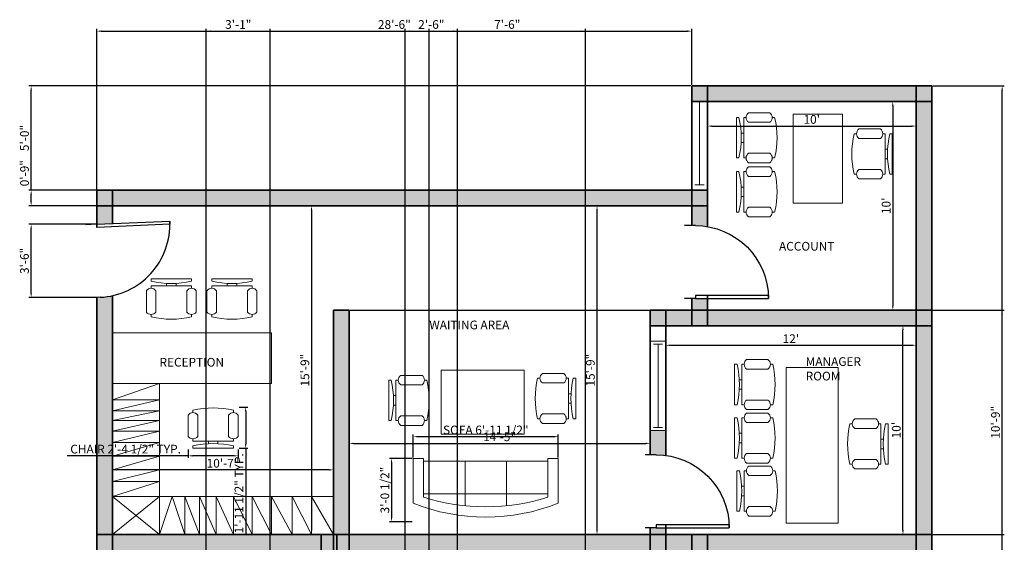
# Model space of a CAD drawing. Units: millimetres. Extents: x 2436 to 3005, y 774 to 1472.
# Tile 3 of 3: x 2436 to 3002, y 1172 to 1472. Entities that reach past the tile are written whole.
import ezdxf

# ---------------------------------------------------------------- set-up
doc = ezdxf.new("R2010")
doc.units = ezdxf.units.MM
for name, color, linetype, lineweight in [('A-ANNO-DIMS', 2, 'Continuous', 18), ('A-AREA-IDEN', 10, 'Continuous', 25), ('A-FLOR-CASE', 140, 'Continuous', 18), ('A-WALL-PATT', 3, 'Continuous', 13), ('doors', 30, 'Continuous', 25), ('furniture', 140, 'Continuous', 18), ('walls', 80, 'Continuous', 35), ('window', 190, 'Continuous', 20)]:
    doc.layers.add(name, color=color, linetype=linetype, lineweight=lineweight)
doc.styles.get("Standard").update_dxf_attribs({"font": 'arial.ttf'})
doc.dimstyles.new('ISO-25', dxfattribs={"dimtxt": 5, "dimasz": 2.5, "dimexe": 1.25, "dimexo": 0.625, "dimtad": 1, "dimdec": 0, "dimlunit": 3, "dimtxsty": 'Standard', "dimcen": 2.5, "dimadec": 0, "dimazin": 0, "dimtfac": 1, "dimtdec": 0, "dimtmove": 0, "dimatfit": 3, "dimfxl": 1, "dimarcsym": 0})

# ---------------------------------------------------------------- blocks, each defined once
blk = doc.blocks.new('*U2')
for p, q in [((0, 0), (0, -6)), ((40, 0), (40, -6))]:
    blk.add_line(p, q)
blk.add_lwpolyline([(0, 0), (0, 40), (1.75, 40), (1.75, 0)], close=True)
blk.add_arc((0, 0), 40, 0, 90)
blk = doc.blocks.new('*U4')
for p, q in [((0, 4), (0, 0)), ((0, 2), (36, 2)), ((36, 4), (36, 0))]:
    blk.add_line(p, q)
blk = doc.blocks.new('Sofa - Roundback 7 ft.')
for p, q in [((-12.00002, -32.4421), (-12.00003, -6.5971)), ((11.99997, -32.4421), (11.99998, -6.5971)), ((-36.000027, -34), (-36.000027, -11.4696)), ((-35.999844, -13.3819), (35.9998, -13.3819)), ((35.99998, -34), (35.99998, -11.4696)), ((-36.000027, -32.4421), (35.99998, -32.4421))]:
    blk.add_line(p, q)
for points in [[(-36.000027, -34), (-42.000027, -34), (-42.000027, -8)], [(41.99998, -8), (41.99998, -34), (35.99998, -34)]]:
    blk.add_lwpolyline(points)
for centre, radius, start, end in [((0, -114.25), 114.25, 68.43141, 111.5686), ((-0.00001, -127.1968), 121.1968, 72.72033, 107.2797)]:
    blk.add_arc(centre, radius, start, end)
blk = doc.blocks.new('Chair - Desk')
for p, q in [((-8.5, 0), (-8.5, -1)), ((-8.5, 0), (8.5, 0)), ((8.5, 0), (8.5, -1)), ((-8.5, -3), (-8.5, -4)), ((-8.5, -3), (8.5, -3)), ((-2, -3), (-2, -1.9355)), ((2, -1.9576), (2, -3)), ((8.5, -3), (8.5, -4)), ((-10.5, -5), (-10.5, -14)), ((-6.5, -14), (-6.5, -5)), ((6.5, -5), (6.5, -14)), ((10.5, -14), (10.5, -5)), ((-8.5, -15), (-8.5, -16)), ((8.5, -15), (8.5, -16))]:
    blk.add_line(p, q)
for centre, radius, start, end in [((-8.5, -6.5), 2.5, 36.8699, 143.1301), ((0, 34.625), 36.625, 256.5803, 283.4197), ((8.5, -6.5), 2.5, 36.8699, 143.1301), ((-8.5, -12.5), 2.5, 216.8699, 323.1301), ((0, 19.625), 36.625, 256.5803, 283.4197), ((8.5, -12.5), 2.5, 216.8699, 323.1301)]:
    blk.add_arc(centre, radius, start, end)
blk = doc.blocks.new('*D9')
at = {"layer": 'A-ANNO-DIMS', "color": 0, "lineweight": -2, "transparency": 16777216}
for p, q in [((2601.07, 1365.12), (2604.93, 1365.12)), ((2603.68, 1362.62), (2603.68, 1178.62)), ((2604.3, 1176.12), (2604.93, 1176.12))]:
    blk.add_line(p, q, dxfattribs=at)
at = {"layer": 'A-ANNO-DIMS', "color": 0, "transparency": 16777216}
for points in [[(2603.26, 1362.62), (2604.09, 1362.62), (2603.68, 1365.12)], [(2603.26, 1178.62), (2604.09, 1178.62), (2603.68, 1176.12)]]:
    blk.add_solid(points, dxfattribs=at)
at = {"layer": 'Defpoints', "color": 0, "transparency": 16777216}
for p in [(2600.44, 1365.12), (2603.68, 1176.12), (2603.68, 1176.12)]:
    blk.add_point(p, dxfattribs=at)
at = {"layer": 'A-ANNO-DIMS', "color": 0, "transparency": 16777216, "insert": (2600.5, 1270.62), "char_height": 5, "attachment_point": 5, "rotation": 90}
blk.add_mtext('15\'-9"', dxfattribs=at)
blk = doc.blocks.new('*D10')
at = {"layer": 'A-ANNO-DIMS', "color": 0, "lineweight": -2, "transparency": 16777216}
for p, q in [((2489.3, 1218.94), (2489.3, 1212.03)), ((2613.8, 1213.28), (2491.8, 1213.28)), ((2616.3, 1215.03), (2616.3, 1212.03))]:
    blk.add_line(p, q, dxfattribs=at)
at = {"layer": 'A-ANNO-DIMS', "color": 0, "transparency": 16777216}
for points in [[(2491.8, 1213.7), (2491.8, 1212.87), (2489.3, 1213.28)], [(2613.8, 1213.7), (2613.8, 1212.87), (2616.3, 1213.28)]]:
    blk.add_solid(points, dxfattribs=at)
at = {"layer": 'Defpoints', "color": 0, "transparency": 16777216}
for p in [(2489.3, 1219.57), (2489.3, 1213.28), (2616.3, 1215.66)]:
    blk.add_point(p, dxfattribs=at)
at = {"layer": 'A-ANNO-DIMS', "color": 0, "transparency": 16777216, "insert": (2552.8, 1216.46), "char_height": 5, "attachment_point": 5}
blk.add_mtext('10\'-7"', dxfattribs=at)
blk = doc.blocks.new('*D11')
at = {"layer": 'A-ANNO-DIMS', "color": 0, "lineweight": -2, "transparency": 16777216}
for p, q in [((2625.3, 1229.12), (2625.3, 1229.75)), ((2627.8, 1228.5), (2795.8, 1228.5)), ((2798.3, 1229.12), (2798.3, 1229.75))]:
    blk.add_line(p, q, dxfattribs=at)
at = {"layer": 'A-ANNO-DIMS', "color": 0, "transparency": 16777216}
for points in [[(2627.8, 1228.91), (2627.8, 1228.08), (2625.3, 1228.5)], [(2795.8, 1228.91), (2795.8, 1228.08), (2798.3, 1228.5)]]:
    blk.add_solid(points, dxfattribs=at)
at = {"layer": 'Defpoints', "color": 0, "transparency": 16777216}
for p in [(2625.3, 1228.5), (2798.3, 1228.5), (2798.3, 1228.5)]:
    blk.add_point(p, dxfattribs=at)
at = {"layer": 'A-ANNO-DIMS', "color": 0, "transparency": 16777216, "insert": (2711.8, 1231.67), "char_height": 5, "attachment_point": 5}
blk.add_mtext('14\'-5"', dxfattribs=at)
blk = doc.blocks.new('*D12')
at = {"layer": 'A-ANNO-DIMS', "color": 0, "lineweight": -2, "transparency": 16777216}
for p, q in [((2773.45, 1365.12), (2766.59, 1365.12)), ((2767.84, 1178.62), (2767.84, 1362.62)), ((2773.45, 1176.12), (2766.59, 1176.12))]:
    blk.add_line(p, q, dxfattribs=at)
at = {"layer": 'A-ANNO-DIMS', "color": 0, "transparency": 16777216}
for points in [[(2767.42, 1362.62), (2768.25, 1362.62), (2767.84, 1365.12)], [(2767.42, 1178.62), (2768.25, 1178.62), (2767.84, 1176.12)]]:
    blk.add_solid(points, dxfattribs=at)
at = {"layer": 'Defpoints', "color": 0, "transparency": 16777216}
for p in [(2767.84, 1365.12), (2774.07, 1365.12), (2774.07, 1176.12)]:
    blk.add_point(p, dxfattribs=at)
at = {"layer": 'A-ANNO-DIMS', "color": 0, "transparency": 16777216, "insert": (2764.66, 1270.62), "char_height": 5, "attachment_point": 5, "rotation": 90}
blk.add_mtext('15\'-9"', dxfattribs=at)
blk = doc.blocks.new('*D13')
at = {"layer": 'A-ANNO-DIMS', "color": 0, "lineweight": -2, "transparency": 16777216}
for p, q in [((2807.3, 1286.74), (2807.3, 1283.69)), ((2951.3, 1286.74), (2951.3, 1283.69)), ((2809.8, 1284.94), (2948.8, 1284.94))]:
    blk.add_line(p, q, dxfattribs=at)
at = {"layer": 'A-ANNO-DIMS', "color": 0, "transparency": 16777216}
for points in [[(2809.8, 1285.36), (2809.8, 1284.53), (2807.3, 1284.94)], [(2948.8, 1285.36), (2948.8, 1284.53), (2951.3, 1284.94)]]:
    blk.add_solid(points, dxfattribs=at)
at = {"layer": 'Defpoints', "color": 0, "transparency": 16777216}
for p in [(2807.3, 1287.36), (2951.3, 1287.36), (2951.3, 1284.94)]:
    blk.add_point(p, dxfattribs=at)
at = {"layer": 'A-ANNO-DIMS', "color": 0, "transparency": 16777216, "insert": (2879.3, 1288.08), "char_height": 5, "attachment_point": 5}
blk.add_mtext("12'", dxfattribs=at)
blk = doc.blocks.new('*D14')
at = {"layer": 'A-ANNO-DIMS', "color": 0, "lineweight": -2, "transparency": 16777216}
for p, q in [((2943.72, 1178.62), (2943.72, 1293.62)), ((2944.34, 1296.12), (2944.97, 1296.12)), ((2944.34, 1176.12), (2944.97, 1176.12))]:
    blk.add_line(p, q, dxfattribs=at)
at = {"layer": 'A-ANNO-DIMS', "color": 0, "transparency": 16777216}
for points in [[(2943.3, 1293.62), (2944.14, 1293.62), (2943.72, 1296.12)], [(2943.3, 1178.62), (2944.14, 1178.62), (2943.72, 1176.12)]]:
    blk.add_solid(points, dxfattribs=at)
at = {"layer": 'Defpoints', "color": 0, "transparency": 16777216}
for p in [(2943.72, 1296.12), (2943.72, 1296.12), (2943.72, 1176.12)]:
    blk.add_point(p, dxfattribs=at)
at = {"layer": 'A-ANNO-DIMS', "color": 0, "transparency": 16777216, "insert": (2940.54, 1236.12), "char_height": 5, "attachment_point": 5, "rotation": 90}
blk.add_mtext("10'", dxfattribs=at)
blk = doc.blocks.new('*D15')
at = {"layer": 'A-ANNO-DIMS', "color": 0, "lineweight": -2, "transparency": 16777216}
for p, q in [((2937.9, 1422.62), (2937.9, 1307.62)), ((2938.53, 1425.12), (2939.15, 1425.12)), ((2938.53, 1305.12), (2939.15, 1305.12))]:
    blk.add_line(p, q, dxfattribs=at)
at = {"layer": 'A-ANNO-DIMS', "color": 0, "transparency": 16777216}
for points in [[(2937.48, 1422.62), (2938.32, 1422.62), (2937.9, 1425.12)], [(2937.48, 1307.62), (2938.32, 1307.62), (2937.9, 1305.12)]]:
    blk.add_solid(points, dxfattribs=at)
at = {"layer": 'Defpoints', "color": 0, "transparency": 16777216}
for p in [(2937.9, 1425.12), (2937.9, 1305.12), (2937.9, 1305.12)]:
    blk.add_point(p, dxfattribs=at)
at = {"layer": 'A-ANNO-DIMS', "color": 0, "transparency": 16777216, "insert": (2934.72, 1365.12), "char_height": 5, "attachment_point": 5, "rotation": 90}
blk.add_mtext("10'", dxfattribs=at)
blk = doc.blocks.new('*D16')
at = {"layer": 'A-ANNO-DIMS', "color": 0, "lineweight": -2, "transparency": 16777216}
for p, q in [((2831.3, 1411.6), (2831.3, 1412.23)), ((2833.8, 1410.98), (2948.8, 1410.98)), ((2951.3, 1411.6), (2951.3, 1412.23))]:
    blk.add_line(p, q, dxfattribs=at)
at = {"layer": 'A-ANNO-DIMS', "color": 0, "transparency": 16777216}
for points in [[(2833.8, 1411.39), (2833.8, 1410.56), (2831.3, 1410.98)], [(2948.8, 1411.39), (2948.8, 1410.56), (2951.3, 1410.98)]]:
    blk.add_solid(points, dxfattribs=at)
at = {"layer": 'Defpoints', "color": 0, "transparency": 16777216}
for p in [(2831.3, 1410.98), (2951.3, 1410.98), (2951.3, 1410.98)]:
    blk.add_point(p, dxfattribs=at)
at = {"layer": 'A-ANNO-DIMS', "color": 0, "transparency": 16777216, "insert": (2891.3, 1414.15), "char_height": 5, "attachment_point": 5}
blk.add_mtext("10'", dxfattribs=at)
blk = doc.blocks.new('*D34')
at = {"layer": 'A-ANNO-DIMS', "color": 0, "lineweight": -2, "transparency": 16777216}
for p, q in [((2532.76, 1225.04), (2532.76, 1220.11)), ((2561.51, 1225.04), (2561.51, 1220.11)), ((2532.76, 1221.36), (2463.27, 1221.36)), ((2559.01, 1221.36), (2535.26, 1221.36))]:
    blk.add_line(p, q, dxfattribs=at)
at = {"layer": 'A-ANNO-DIMS', "color": 0, "transparency": 16777216}
for points in [[(2535.26, 1221.77), (2535.26, 1220.94), (2532.76, 1221.36)], [(2559.01, 1221.77), (2559.01, 1220.94), (2561.51, 1221.36)]]:
    blk.add_solid(points, dxfattribs=at)
at = {"layer": 'Defpoints', "color": 0, "transparency": 16777216}
for p in [(2532.76, 1225.67), (2561.51, 1225.67), (2532.76, 1221.36)]:
    blk.add_point(p, dxfattribs=at)
at = {"layer": 'A-ANNO-DIMS', "color": 0, "transparency": 16777216, "insert": (2496.77, 1224.57), "char_height": 5, "attachment_point": 5}
blk.add_mtext('CHAIR 2\'-4 1/2" TYP.', dxfattribs=at)
blk = doc.blocks.new('*D35')
at = {"layer": 'A-ANNO-DIMS', "color": 0, "lineweight": -2, "transparency": 16777216}
for p, q in [((2562.13, 1249.39), (2567.07, 1249.39)), ((2565.82, 1246.89), (2565.82, 1228.17)), ((2562.13, 1225.67), (2567.07, 1225.67)), ((2565.82, 1225.67), (2565.82, 1176.38))]:
    blk.add_line(p, q, dxfattribs=at)
at = {"layer": 'A-ANNO-DIMS', "color": 0, "transparency": 16777216}
for points in [[(2565.4, 1246.89), (2566.23, 1246.89), (2565.82, 1249.39)], [(2565.4, 1228.17), (2566.23, 1228.17), (2565.82, 1225.67)]]:
    blk.add_solid(points, dxfattribs=at)
at = {"layer": 'Defpoints', "color": 0, "transparency": 16777216}
for p in [(2561.51, 1249.39), (2561.51, 1225.67), (2565.82, 1225.67)]:
    blk.add_point(p, dxfattribs=at)
at = {"layer": 'A-ANNO-DIMS', "color": 0, "transparency": 16777216, "insert": (2562.61, 1199.77), "char_height": 5, "attachment_point": 5, "rotation": 90}
blk.add_mtext('1\'-11 1/2" TYP.', dxfattribs=at)
blk = doc.blocks.new('*D38')
at = {"layer": 'A-ANNO-DIMS', "color": 0, "lineweight": -2, "transparency": 16777216}
for p, q in [((2662.2, 1220.49), (2662.2, 1233.62)), ((2743.04, 1232.37), (2664.7, 1232.37)), ((2745.54, 1220.49), (2745.54, 1233.62))]:
    blk.add_line(p, q, dxfattribs=at)
at = {"layer": 'A-ANNO-DIMS', "color": 0, "transparency": 16777216}
for points in [[(2664.7, 1232.79), (2664.7, 1231.95), (2662.2, 1232.37)], [(2743.04, 1232.79), (2743.04, 1231.95), (2745.54, 1232.37)]]:
    blk.add_solid(points, dxfattribs=at)
at = {"layer": 'Defpoints', "color": 0, "transparency": 16777216}
for p in [(2662.2, 1232.37), (2662.2, 1219.87), (2745.54, 1219.87)]:
    blk.add_point(p, dxfattribs=at)
at = {"layer": 'A-ANNO-DIMS', "color": 0, "transparency": 16777216, "insert": (2703.87, 1235.58), "char_height": 5, "attachment_point": 5}
blk.add_mtext('SOFA 6\'-11 1/2"', dxfattribs=at)
blk = doc.blocks.new('*D39')
at = {"layer": 'A-ANNO-DIMS', "color": 0, "lineweight": -2, "transparency": 16777216}
for p, q in [((2661.57, 1219.87), (2648.45, 1219.87)), ((2649.7, 1217.37), (2649.7, 1185.99)), ((2661.57, 1183.49), (2648.45, 1183.49))]:
    blk.add_line(p, q, dxfattribs=at)
at = {"layer": 'A-ANNO-DIMS', "color": 0, "transparency": 16777216}
for points in [[(2649.28, 1217.37), (2650.11, 1217.37), (2649.7, 1219.87)], [(2649.28, 1185.99), (2650.11, 1185.99), (2649.7, 1183.49)]]:
    blk.add_solid(points, dxfattribs=at)
at = {"layer": 'Defpoints', "color": 0, "transparency": 16777216}
for p in [(2662.2, 1219.87), (2649.7, 1183.49), (2662.2, 1183.49)]:
    blk.add_point(p, dxfattribs=at)
at = {"layer": 'A-ANNO-DIMS', "color": 0, "transparency": 16777216, "insert": (2646.48, 1201.68), "char_height": 5, "attachment_point": 5, "rotation": 90}
blk.add_mtext('3\'-0 1/2"', dxfattribs=at)
blk = doc.blocks.new('*D41')
at = {"layer": 'A-ANNO-DIMS', "color": 0, "lineweight": -2, "transparency": 16777216}
for p, q in [((2960.92, 1434.12), (3002, 1434.12)), ((3000.75, 809.62), (3000.75, 1431.62)), ((2969.92, 807.12), (3002, 807.12))]:
    blk.add_line(p, q, dxfattribs=at)
at = {"layer": 'A-ANNO-DIMS', "color": 0, "transparency": 16777216}
for points in [[(3000.33, 1431.62), (3001.17, 1431.62), (3000.75, 1434.12)], [(3000.33, 809.62), (3001.17, 809.62), (3000.75, 807.12)]]:
    blk.add_solid(points, dxfattribs=at)
at = {"layer": 'Defpoints', "color": 0, "transparency": 16777216}
for p in [(2960.3, 1434.12), (3000.75, 1434.12), (2969.3, 807.12)]:
    blk.add_point(p, dxfattribs=at)
at = {"layer": 'A-ANNO-DIMS', "color": 0, "transparency": 16777216, "insert": (2997.57, 1120.62), "char_height": 5, "attachment_point": 5, "rotation": 90}
blk.add_mtext('52\'-3"', dxfattribs=at)
blk = doc.blocks.new('*D43')
at = {"layer": 'A-ANNO-DIMS', "color": 0, "lineweight": -2, "transparency": 16777216}
for p, q in [((2822.3, 1175.5), (2822.3, 774.42)), ((2618.3, 1160.31), (2618.3, 774.42)), ((2620.8, 775.67), (2819.8, 775.67))]:
    blk.add_line(p, q, dxfattribs=at)
at = {"layer": 'A-ANNO-DIMS', "color": 0, "transparency": 16777216}
for points in [[(2620.8, 776.09), (2620.8, 775.26), (2618.3, 775.67)], [(2819.8, 776.09), (2819.8, 775.26), (2822.3, 775.67)]]:
    blk.add_solid(points, dxfattribs=at)
at = {"layer": 'Defpoints', "color": 0, "transparency": 16777216}
for p in [(2822.3, 1176.12), (2618.3, 1160.93), (2822.3, 775.67)]:
    blk.add_point(p, dxfattribs=at)
at = {"layer": 'A-ANNO-DIMS', "color": 0, "transparency": 16777216, "insert": (2720.3, 778.85), "char_height": 5, "attachment_point": 5}
blk.add_mtext('17\'-0"', dxfattribs=at)
blk = doc.blocks.new('*D45')
at = {"layer": 'A-ANNO-DIMS', "color": 0, "lineweight": -2, "transparency": 16777216}
for p, q in [((2480.3, 1374.75), (2480.3, 1466.82)), ((2822.3, 1434.75), (2822.3, 1466.82)), ((2482.8, 1465.57), (2819.8, 1465.57))]:
    blk.add_line(p, q, dxfattribs=at)
at = {"layer": 'A-ANNO-DIMS', "color": 0, "transparency": 16777216}
for points in [[(2482.8, 1465.99), (2482.8, 1465.16), (2480.3, 1465.57)], [(2819.8, 1465.99), (2819.8, 1465.16), (2822.3, 1465.57)]]:
    blk.add_solid(points, dxfattribs=at)
at = {"layer": 'Defpoints', "color": 0, "transparency": 16777216}
for p in [(2822.3, 1465.57), (2822.3, 1434.12), (2480.3, 1374.12)]:
    blk.add_point(p, dxfattribs=at)
at = {"layer": 'A-ANNO-DIMS', "color": 0, "transparency": 16777216, "insert": (2651.3, 1468.75), "char_height": 5, "attachment_point": 5}
blk.add_mtext('28\'-6"', dxfattribs=at)
blk = doc.blocks.new('*D46')
at = {"layer": 'A-ANNO-DIMS', "color": 0, "lineweight": -2, "transparency": 16777216}
for p, q in [((2821.67, 1434.12), (2441.22, 1434.12)), ((2442.47, 1376.62), (2442.47, 1431.62)), ((2830.67, 1374.12), (2441.22, 1374.12))]:
    blk.add_line(p, q, dxfattribs=at)
at = {"layer": 'A-ANNO-DIMS', "color": 0, "transparency": 16777216}
for points in [[(2442.06, 1431.62), (2442.89, 1431.62), (2442.47, 1434.12)], [(2442.06, 1376.62), (2442.89, 1376.62), (2442.47, 1374.12)]]:
    blk.add_solid(points, dxfattribs=at)
at = {"layer": 'Defpoints', "color": 0, "transparency": 16777216}
for p in [(2442.47, 1434.12), (2822.3, 1434.12), (2831.3, 1374.12)]:
    blk.add_point(p, dxfattribs=at)
at = {"layer": 'A-ANNO-DIMS', "color": 0, "transparency": 16777216, "insert": (2439.29, 1404.12), "char_height": 5, "attachment_point": 5, "rotation": 90}
blk.add_mtext('5\'-0"', dxfattribs=at)
blk = doc.blocks.new('*D47')
at = {"layer": 'A-ANNO-DIMS', "color": 0, "lineweight": -2, "transparency": 16777216}
for p, q in [((2479.59, 1354.48), (2441.22, 1354.48)), ((2442.47, 1314.94), (2442.47, 1351.98)), ((2479.67, 1312.44), (2441.22, 1312.44))]:
    blk.add_line(p, q, dxfattribs=at)
at = {"layer": 'A-ANNO-DIMS', "color": 0, "transparency": 16777216}
for points in [[(2442.06, 1351.98), (2442.89, 1351.98), (2442.47, 1354.48)], [(2442.06, 1314.94), (2442.89, 1314.94), (2442.47, 1312.44)]]:
    blk.add_solid(points, dxfattribs=at)
at = {"layer": 'Defpoints', "color": 0, "transparency": 16777216}
for p in [(2442.47, 1354.48), (2480.22, 1354.48), (2480.3, 1312.44)]:
    blk.add_point(p, dxfattribs=at)
at = {"layer": 'A-ANNO-DIMS', "color": 0, "transparency": 16777216, "insert": (2439.29, 1333.46), "char_height": 5, "attachment_point": 5, "rotation": 90}
blk.add_mtext('3\'-6"', dxfattribs=at)
blk = doc.blocks.new('*D48')
at = {"layer": 'A-ANNO-DIMS', "color": 0, "lineweight": -2, "transparency": 16777216}
for p, q in [((2442.47, 1374.12), (2442.47, 1391.16)), ((2479.67, 1374.12), (2441.22, 1374.12)), ((2442.47, 1367.62), (2442.47, 1371.62)), ((2479.67, 1365.12), (2441.22, 1365.12))]:
    blk.add_line(p, q, dxfattribs=at)
at = {"layer": 'A-ANNO-DIMS', "color": 0, "transparency": 16777216}
for points in [[(2442.06, 1371.62), (2442.89, 1371.62), (2442.47, 1374.12)], [(2442.06, 1367.62), (2442.89, 1367.62), (2442.47, 1365.12)]]:
    blk.add_solid(points, dxfattribs=at)
at = {"layer": 'Defpoints', "color": 0, "transparency": 16777216}
for p in [(2442.47, 1374.12), (2480.3, 1374.12), (2480.3, 1365.12)]:
    blk.add_point(p, dxfattribs=at)
at = {"layer": 'A-ANNO-DIMS', "color": 0, "transparency": 16777216, "insert": (2439.29, 1383.89), "char_height": 5, "attachment_point": 5, "rotation": 90}
blk.add_mtext('0\'-9"', dxfattribs=at)
blk = doc.blocks.new('*D49')
at = {"layer": 'A-ANNO-DIMS', "color": 0, "lineweight": -2, "transparency": 16777216}
for p, q in [((2671.31, 1103.79), (2671.31, 1466.82)), ((2761.12, 1103.79), (2761.12, 1466.82)), ((2673.81, 1465.57), (2758.62, 1465.57))]:
    blk.add_line(p, q, dxfattribs=at)
at = {"layer": 'A-ANNO-DIMS', "color": 0, "transparency": 16777216}
for points in [[(2673.81, 1465.99), (2673.81, 1465.16), (2671.31, 1465.57)], [(2758.62, 1465.99), (2758.62, 1465.16), (2761.12, 1465.57)]]:
    blk.add_solid(points, dxfattribs=at)
at = {"layer": 'Defpoints', "color": 0, "transparency": 16777216}
for p in [(2761.12, 1465.57), (2671.31, 1103.17), (2761.12, 1103.17)]:
    blk.add_point(p, dxfattribs=at)
at = {"layer": 'A-ANNO-DIMS', "color": 0, "transparency": 16777216, "insert": (2716.21, 1468.75), "char_height": 5, "attachment_point": 5}
blk.add_mtext('7\'-6"', dxfattribs=at)
blk = doc.blocks.new('*D51')
at = {"layer": 'A-ANNO-DIMS', "color": 0, "lineweight": -2, "transparency": 16777216}
for p, q in [((2625.92, 1305.12), (3002, 1305.12)), ((3000.75, 1178.62), (3000.75, 1302.62)), ((2618.92, 1176.12), (3002, 1176.12))]:
    blk.add_line(p, q, dxfattribs=at)
at = {"layer": 'A-ANNO-DIMS', "color": 0, "transparency": 16777216}
for points in [[(3000.33, 1302.62), (3001.17, 1302.62), (3000.75, 1305.12)], [(3000.33, 1178.62), (3001.17, 1178.62), (3000.75, 1176.12)]]:
    blk.add_solid(points, dxfattribs=at)
at = {"layer": 'Defpoints', "color": 0, "transparency": 16777216}
for p in [(2625.3, 1305.12), (3000.75, 1305.12), (2618.3, 1176.12)]:
    blk.add_point(p, dxfattribs=at)
at = {"layer": 'A-ANNO-DIMS', "color": 0, "transparency": 16777216, "insert": (2997.57, 1240.62), "char_height": 5, "attachment_point": 5, "rotation": 90}
blk.add_mtext('10\'-9"', dxfattribs=at)
blk = doc.blocks.new('*D52')
at = {"layer": 'A-ANNO-DIMS', "color": 0, "lineweight": -2, "transparency": 16777216}
for p, q in [((2657.55, 932.75), (2657.55, 1466.82)), ((2687.55, 932.75), (2687.55, 1466.82)), ((2660.05, 1465.57), (2685.05, 1465.57))]:
    blk.add_line(p, q, dxfattribs=at)
at = {"layer": 'A-ANNO-DIMS', "color": 0, "transparency": 16777216}
for points in [[(2660.05, 1465.99), (2660.05, 1465.16), (2657.55, 1465.57)], [(2685.05, 1465.99), (2685.05, 1465.16), (2687.55, 1465.57)]]:
    blk.add_solid(points, dxfattribs=at)
at = {"layer": 'Defpoints', "color": 0, "transparency": 16777216}
for p in [(2687.55, 1465.57), (2657.55, 932.12), (2687.55, 932.12)]:
    blk.add_point(p, dxfattribs=at)
at = {"layer": 'A-ANNO-DIMS', "color": 0, "transparency": 16777216, "insert": (2672.55, 1468.75), "char_height": 5, "attachment_point": 5}
blk.add_mtext('2\'-6"', dxfattribs=at)
blk = doc.blocks.new('*D53')
at = {"layer": 'A-ANNO-DIMS', "color": 0, "lineweight": -2, "transparency": 16777216}
for p, q in [((2543.16, 945.65), (2543.16, 1466.82)), ((2579.92, 945.65), (2579.92, 1466.82)), ((2545.66, 1465.57), (2577.42, 1465.57))]:
    blk.add_line(p, q, dxfattribs=at)
at = {"layer": 'A-ANNO-DIMS', "color": 0, "transparency": 16777216}
for points in [[(2545.66, 1465.99), (2545.66, 1465.16), (2543.16, 1465.57)], [(2577.42, 1465.99), (2577.42, 1465.16), (2579.92, 1465.57)]]:
    blk.add_solid(points, dxfattribs=at)
at = {"layer": 'Defpoints', "color": 0, "transparency": 16777216}
for p in [(2579.92, 1465.57), (2543.16, 945.02), (2579.92, 945.02)]:
    blk.add_point(p, dxfattribs=at)
at = {"layer": 'A-ANNO-DIMS', "color": 0, "transparency": 16777216, "insert": (2561.54, 1468.75), "char_height": 5, "attachment_point": 5}
blk.add_mtext('3\'-1"', dxfattribs=at)

msp = doc.modelspace()

# ---------------------------------------------------------------- hatches: boundary and pattern name
at = {"layer": 'A-WALL-PATT'}
h = msp.add_hatch(color=256, dxfattribs=at)
h.dxf.hatch_style = 1
h.paths.add_polyline_path([(2822.3, 1374.12), (2489.3, 1374.12), (2489.3, 1365.12), (2822.3, 1365.12)])
h.paths.add_polyline_path([(2831.3, 1374.12), (2822.3, 1374.12), (2822.3, 1365.12), (2831.3, 1365.12)])
h.paths.add_polyline_path([(2831.3, 1365.12), (2822.3, 1365.12), (2822.3, 1353.75), (2824.37, 1353.75, -0.041466), (2831.3, 1353.17)])
h.paths.add_polyline_path([(2960.3, 1425.12), (2951.3, 1425.12), (2951.3, 1305.12), (2960.3, 1305.12)])
h.paths.add_polyline_path([(2960.3, 1434.12), (2951.3, 1434.12), (2951.3, 1425.12), (2960.3, 1425.12)])
h.paths.add_polyline_path([(2951.3, 1434.12), (2831.3, 1434.12), (2831.3, 1425.12), (2951.3, 1425.12)])
h.paths.add_polyline_path([(2831.3, 1434.12), (2822.3, 1434.12), (2822.3, 1425.12), (2831.3, 1425.12)])
h.paths.add_polyline_path([(2489.3, 1374.12), (2480.3, 1374.12), (2480.3, 1365.12), (2489.3, 1365.12)])
h.paths.add_polyline_path([(2489.3, 1365.12), (2480.3, 1365.12), (2480.3, 1354.49), (2489.3, 1354.89)])
h.paths.add_polyline_path([(2489.3, 1313.48, -0.04329), (2482.1, 1312.53), (2480.3, 1312.44), (2480.3, 1176.12), (2489.3, 1176.12)])
h.paths.add_polyline_path([(2489.3, 1176.12), (2480.3, 1176.12), (2480.3, 1167.12), (2489.3, 1167.12)])
h.paths.add_polyline_path([(2609.3, 1176.12), (2489.3, 1176.12), (2489.3, 1167.12), (2609.3, 1167.12)])
h.paths.add_polyline_path([(2625.3, 1176.12), (2618.3, 1176.12), (2618.3, 1167.12), (2625.3, 1167.12)])
h.paths.add_polyline_path([(2618.3, 1176.12), (2616.3, 1176.12), (2616.3, 1167.12), (2618.3, 1167.12)])
h.paths.add_polyline_path([(2616.3, 1176.12), (2609.3, 1176.12), (2609.3, 1167.12), (2616.3, 1167.12)])
h.paths.add_polyline_path([(2618.3, 1167.12), (2609.3, 1167.12), (2609.3, 1160.63, -0.029892), (2614.31, 1160.93), (2618.3, 1160.93)])
h.paths.add_polyline_path([(2625.3, 1305.12), (2616.3, 1305.12), (2616.3, 1176.12), (2618.3, 1176.12), (2625.3, 1176.12)])
h.paths.add_polyline_path([(2798.3, 1176.12), (2625.3, 1176.12), (2625.3, 1167.12), (2798.3, 1167.12)])
h.paths.add_polyline_path([(2807.3, 1176.12), (2798.3, 1176.12), (2798.3, 1167.12), (2807.3, 1167.12)])
h.paths.add_polyline_path([(2831.3, 1176.12), (2822.3, 1176.12), (2822.3, 1167.12), (2831.3, 1167.12)])
h.paths.add_polyline_path([(2822.3, 1176.12), (2807.3, 1176.12), (2807.3, 1167.12), (2822.3, 1167.12)])
h.paths.add_polyline_path([(2951.3, 1176.12), (2831.3, 1176.12), (2831.3, 1167.12), (2951.3, 1167.12)])
h.paths.add_polyline_path([(2960.3, 1176.12), (2951.3, 1176.12), (2951.3, 1167.12), (2960.3, 1167.12)])
h.paths.add_polyline_path([(2960.3, 1296.12), (2951.3, 1296.12), (2951.3, 1176.12), (2960.3, 1176.12)])
h.paths.add_polyline_path([(2960.3, 1305.12), (2951.3, 1305.12), (2951.3, 1296.12), (2960.3, 1296.12)])
h.paths.add_polyline_path([(2951.3, 1305.12), (2831.3, 1305.12), (2831.3, 1296.12), (2951.3, 1296.12)])
h.paths.add_polyline_path([(2822.3, 1305.12), (2807.3, 1305.12), (2807.3, 1296.12), (2822.3, 1296.12)])
h.paths.add_polyline_path([(2831.3, 1305.12), (2822.3, 1305.12), (2822.3, 1296.12), (2831.3, 1296.12)])
h.paths.add_polyline_path([(2831.3, 1311.75), (2824.37, 1311.75), (2822.3, 1311.75), (2822.3, 1305.12), (2831.3, 1305.12)])
h.paths.add_polyline_path([(2807.3, 1305.12), (2798.3, 1305.12), (2798.3, 1296.12), (2807.3, 1296.12)])
h.paths.add_polyline_path([(2807.3, 1236.01), (2798.3, 1236.01), (2798.3, 1221.93), (2801.81, 1221.93, -0.032777), (2807.3, 1221.57)])
h.paths.add_polyline_path([(2831.3, 1167.12), (2822.3, 1167.12), (2822.3, 1139.2), (2826.09, 1139.2, -0.043681), (2831.3, 1138.75)])
h.paths.add_polyline_path([(2807.3, 1179.93), (2801.81, 1179.93), (2798.3, 1179.93), (2798.3, 1176.12), (2807.3, 1176.12)])
h.paths.add_polyline_path([(2927.3, 900.12), (2831.3, 900.12), (2831.3, 891.12), (2927.3, 891.12)])
h.paths.add_polyline_path([(2936.3, 900.12), (2927.3, 900.12), (2927.3, 891.12), (2936.3, 891.12)])
h.paths.add_polyline_path([(2936.3, 905.69), (2927.3, 905.69), (2927.3, 900.12), (2936.3, 900.12)])
h.paths.add_polyline_path([(2831.3, 900.12), (2822.3, 900.12), (2822.3, 891.12), (2831.3, 891.12)])
h.paths.add_polyline_path([(2831.3, 903.84), (2822.3, 903.84), (2822.3, 900.12), (2831.3, 900.12)])
h.paths.add_polyline_path([(2822.3, 900.12), (2812.6, 900.12), (2812.6, 896.54), (2812.6, 891.12), (2822.3, 891.12)])
h.paths.add_polyline_path([(2969.3, 900.12), (2958.95, 900.12), (2936.3, 900.12), (2936.3, 891.12), (2960.3, 891.12), (2960.3, 826.87), (2960.3, 816.12), (2969.3, 816.12), (2969.3, 826.87), (2969.3, 891.12)])

# ---------------------------------------------------------------- linework, layer by layer
at = {"layer": 'A-FLOR-CASE'}
for p, q in [((2489.3, 1253.53), (2516.31, 1263.01)), ((2516.31, 1263.01), (2489.3, 1263.01)), ((2489.3, 1247.21), (2516.31, 1253.53)), ((2516.31, 1253.53), (2489.3, 1253.53)), ((2489.3, 1241.6), (2516.31, 1247.21)), ((2516.31, 1247.21), (2489.3, 1247.21)), ((2489.3, 1235.46), (2516.31, 1241.6)), ((2516.31, 1241.6), (2489.3, 1241.6)), ((2489.3, 1229), (2516.31, 1235.46)), ((2516.31, 1235.46), (2489.3, 1235.46)), ((2489.3, 1221.2), (2516.31, 1229)), ((2516.31, 1229), (2489.3, 1229)), ((2489.3, 1213.28), (2516.31, 1221.2)), ((2516.31, 1221.2), (2489.3, 1221.2)), ((2489.3, 1206.56), (2516.31, 1213.28)), ((2516.31, 1213.28), (2489.3, 1213.28)), ((2489.3, 1197.98), (2516.31, 1206.56)), ((2516.31, 1206.56), (2489.3, 1206.56)), ((2516.31, 1176.12), (2489.3, 1197.98)), ((2489.3, 1197.98), (2516.31, 1197.98)), ((2516.31, 1197.98), (2489.3, 1176.12)), ((2523.48, 1197.98), (2516.31, 1176.12)), ((2530.89, 1176.12), (2523.48, 1197.98)), ((2539.35, 1176.12), (2530.89, 1197.98)), ((2530.89, 1197.98), (2530.89, 1176.12)), ((2548.88, 1176.12), (2539.35, 1197.98)), ((2539.35, 1197.98), (2539.35, 1176.12)), ((2558.81, 1176.12), (2548.88, 1197.98)), ((2548.88, 1197.98), (2548.88, 1176.12)), ((2569.56, 1176.12), (2558.81, 1197.98)), ((2558.81, 1197.98), (2558.81, 1176.12)), ((2580.63, 1176.12), (2569.56, 1197.98)), ((2569.56, 1197.98), (2569.56, 1176.12)), ((2592.52, 1176.12), (2580.63, 1197.98)), ((2580.63, 1197.98), (2580.63, 1176.12)), ((2603.68, 1176.12), (2592.52, 1197.98)), ((2592.52, 1197.98), (2592.52, 1176.12)), ((2616.3, 1176.12), (2603.68, 1197.98)), ((2603.68, 1197.98), (2603.68, 1176.12))]:
    msp.add_line(p, q, dxfattribs=at)
for points in [[(2489.3, 1263.01), (2580.59, 1263.01), (2580.59, 1292.14), (2489.3, 1292.14)], [(2489.3, 1176.12), (2516.31, 1176.12), (2516.31, 1263.01), (2489.3, 1263.01)], [(2616.3, 1176.12), (2489.3, 1176.12), (2489.3, 1197.98), (2616.3, 1197.98)]]:
    msp.add_lwpolyline(points, close=True, dxfattribs=at)
at = {"layer": 'furniture'}
for points in [[(2880.58, 1417.84), (2908.9, 1417.84), (2908.9, 1366.74), (2880.58, 1366.74)], [(2678.31, 1270.53), (2725.92, 1270.53), (2725.92, 1233.86), (2678.31, 1233.86)], [(2876.66, 1272.17), (2906.45, 1272.17), (2906.45, 1182.62), (2876.66, 1182.62)]]:
    msp.add_lwpolyline(points, close=True, dxfattribs=at)
at = {"layer": 'walls'}
for p, q in [((2960.3, 1434.12), (2822.3, 1434.12)), ((2822.3, 1434.12), (2822.3, 1353.75)), ((2822.3, 1434.12), (2822.3, 1386.13)), ((2960.3, 1434.12), (2822.3, 1434.12)), ((2822.3, 1434.12), (2822.3, 1353.75)), ((2831.3, 1434.12), (2831.3, 1353.17)), ((2831.3, 1434.12), (2831.3, 1353.17)), ((2951.3, 1434.12), (2951.3, 1098.12)), ((2960.3, 1434.12), (2960.3, 1098.12)), ((2960.3, 1425.12), (2822.3, 1425.12)), ((2480.3, 1374.12), (2480.3, 1352.65)), ((2831.3, 1374.12), (2480.3, 1374.12)), ((2489.3, 1374.12), (2489.3, 1354.89)), ((2831.3, 1365.12), (2480.3, 1365.12)), ((2489.3, 1313.48), (2489.3, 807.12)), ((2831.3, 1313.59), (2831.3, 1296.12)), ((2831.3, 1313.59), (2831.3, 1296.12)), ((2480.3, 1312.44), (2480.3, 807.12)), ((2822.3, 1311.75), (2822.3, 1296.12)), ((2822.3, 1311.75), (2822.3, 1296.12)), ((2616.3, 1305.12), (2616.3, 1167.12)), ((2625.3, 1305.12), (2616.3, 1305.12)), ((2625.3, 1305.12), (2625.3, 1167.12)), ((2960.3, 1305.12), (2798.3, 1305.12)), ((2798.3, 1305.12), (2798.3, 1221.93)), ((2807.3, 1305.12), (2807.3, 1221.57)), ((2960.3, 1296.12), (2798.3, 1296.12)), ((2798.3, 1179.93), (2798.3, 1167.12)), ((2807.3, 1181.77), (2807.3, 1167.12)), ((2960.3, 1176.12), (2480.3, 1176.12)), ((2609.3, 1176.12), (2609.3, 1160.63)), ((2618.3, 1176.12), (2618.3, 1160.93)), ((2822.3, 1176.12), (2822.3, 1139.2)), ((2831.3, 1176.12), (2831.3, 1138.75))]:
    msp.add_line(p, q, dxfattribs=at)
at = {"layer": 'window'}
for p, q in [((2807.3, 1287.36), (2798.3, 1287.36)), ((2798.3, 1236.01), (2807.3, 1236.01))]:
    msp.add_line(p, q, dxfattribs=at)

# ---------------------------------------------------------------- block references
at = {"layer": 'doors'}
for p, xscale, yscale, zscale, rotation in [((2480.22, 1354.48), 1.049999999999999, 1.049999999999999, 1.049999999999999, 272.5737265513209), ((2824.37, 1311.75), -1.05, 1.05, 1.05, 270), ((2801.81, 1179.93), -1.05, 1.05, 1.05, 270)]:
    msp.add_blockref('*U2', p, dxfattribs=dict(at, xscale=xscale, yscale=yscale, zscale=zscale, rotation=rotation))
at = {"layer": 'furniture'}
for name, p, xscale, yscale, zscale, rotation in [('Chair - Desk', (2848.05, 1404.26), 1.368662376549279, 1.368662376549279, 1.368662376549279, 90), ('Chair - Desk', (2937.57, 1394.96), 1.368662376549279, 1.368662376549279, 1.368662376549279, 270), ('Chair - Desk', (2848.05, 1373.17), 1.368662376549279, 1.368662376549279, 1.368662376549279, 90), ('Chair - Desk', (2846.96, 1262.35), 1.368662376549279, 1.368662376549279, 1.368662376549279, 90), ('Chair - Desk', (2755.57, 1254.34), 1.368662376549279, 1.368662376549279, 1.368662376549279, 270), ('Chair - Desk', (2648.09, 1253.26), 1.368662376549279, 1.368662376549279, 1.368662376549279, 90), ('Chair - Desk', (2547.13, 1225.67), 1.368662376549279, 1.368662376549279, 1.368662376549279, 180), ('Chair - Desk', (2846.96, 1231.58), 1.368662376549279, 1.368662376549279, 1.368662376549279, 90), ('Chair - Desk', (2935.14, 1228.21), 1.368662376549279, 1.368662376549279, 1.368662376549279, 270), ('Sofa - Roundback 7 ft.', (2703.87, 1186.14), 0.9921543039801486, 0.9921543039801486, 0.9921543039801486, 180), ('Chair - Desk', (2848.29, 1201.12), 1.368662376549279, 1.368662376549279, 1.368662376549279, 90)]:
    msp.add_blockref(name, p, dxfattribs=dict(at, xscale=xscale, yscale=yscale, zscale=zscale, rotation=rotation))
at = {"layer": 'furniture', "xscale": 1.368662376549279, "yscale": 1.368662376549279, "zscale": 1.368662376549279}
for p in [(2523.07, 1323.17), (2557.93, 1323.17)]:
    msp.add_blockref('Chair - Desk', p, dxfattribs=at)
at = {"layer": 'window', "xscale": 1.333333333333333, "yscale": 1.333333333333333, "zscale": 1.333333333333333, "rotation": 90}
for p in [(2829.4, 1377.12), (2805.56, 1237.65)]:
    msp.add_blockref('*U4', p, dxfattribs=at)

# ---------------------------------------------------------------- texts
at = {"layer": 'A-AREA-IDEN', "char_height": 5, "attachment_point": 1}
for s, width, insert in [('ACCOUNT ', 47.0426, (2872.46, 1344.36)), ('WAITING AREA', 73.0525, (2671.41, 1299.13)), ('RECEPTION', 43.6196, (2516.26, 1277.67)), ('MANAGER ROOM', 23.8883, (2887.79, 1278.06))]:
    msp.add_mtext_dynamic_manual_height_columns(s, width=width, gutter_width=12.5, heights=[0], dxfattribs=dict(at, insert=insert))

# ---------------------------------------------------------------- dimensions: what is measured, and where the dimension line sits
at = {"layer": 'A-ANNO-DIMS'}
for base, p1, p2, override, picture, middle in [((2822.3, 1465.57), (2480.3, 1374.12), (2822.3, 1434.12), {"dimdec": 1, "dimlfac": 1, "dimrnd": 0, "dimzin": 1, "dimdsep": 46, "dimlunit": 4, "dimfrac": 2}, '*D45', (2651.3, 1468.75)), ((2579.92, 1465.57), (2543.16, 945.02), (2579.92, 945.02), {"dimdec": 1, "dimlfac": 1, "dimrnd": 0, "dimzin": 1, "dimdsep": 46, "dimlunit": 4, "dimfrac": 2}, '*D53', (2561.54, 1468.75)), ((2687.55, 1465.57), (2657.55, 932.12), (2687.55, 932.12), {"dimdec": 1, "dimlfac": 1, "dimrnd": 0, "dimzin": 1, "dimdsep": 46, "dimlunit": 4, "dimfrac": 2}, '*D52', (2672.55, 1468.75)), ((2761.12, 1465.57), (2671.31, 1103.17), (2761.12, 1103.17), {"dimdec": 1, "dimlfac": 1, "dimrnd": 0, "dimzin": 1, "dimdsep": 46, "dimlunit": 4, "dimfrac": 2}, '*D49', (2716.21, 1468.75)), ((2951.3, 1410.98), (2831.3, 1410.98), (2951.3, 1410.98), {"dimclrd": 0, "dimclre": 0, "dimclrt": 0}, '*D16', (2891.3, 1414.15)), ((2951.3, 1284.94), (2807.3, 1287.36), (2951.3, 1287.36), {"dimclrd": 0, "dimclre": 0, "dimclrt": 0}, '*D13', (2879.3, 1288.08)), ((2798.3, 1228.5), (2625.3, 1228.5), (2798.3, 1228.5), {"dimclrd": 0, "dimclre": 0, "dimclrt": 0}, '*D11', (2711.8, 1231.67)), ((2489.3, 1213.28), (2616.3, 1215.66), (2489.3, 1219.57), {"dimclrd": 0, "dimclre": 0, "dimclrt": 0}, '*D10', (2552.8, 1216.46)), ((2822.3, 775.67), (2618.3, 1160.93), (2822.3, 1176.12), {"dimdec": 1, "dimlfac": 1, "dimrnd": 0, "dimzin": 1, "dimdsep": 46, "dimlunit": 4, "dimfrac": 2}, '*D43', (2720.3, 778.85))]:
    dim = msp.add_linear_dim(base=base, p1=p1, p2=p2, dimstyle='ISO-25', override=override, dxfattribs=at)
    dim.commit()
    dim.dimension.update_dxf_attribs({"geometry": picture, "text_midpoint": middle})
for base, p1, p2, angle, override, picture, middle in [((2442.47, 1434.12), (2831.3, 1374.12), (2822.3, 1434.12), 90, {"dimdec": 1, "dimlfac": 1, "dimrnd": 0, "dimzin": 1, "dimdsep": 46, "dimlunit": 4, "dimfrac": 2}, '*D46', (2439.29, 1404.12)), ((3000.75, 1434.12), (2969.3, 807.12), (2960.3, 1434.12), 90, {"dimdec": 1, "dimlfac": 1, "dimrnd": 0, "dimzin": 1, "dimdsep": 46, "dimlunit": 4, "dimfrac": 2}, '*D41', (2997.57, 1120.62)), ((2937.9, 1305.12), (2937.9, 1425.12), (2937.9, 1305.12), 90, {"dimclrd": 0, "dimclre": 0, "dimclrt": 0}, '*D15', (2934.72, 1365.12)), ((2442.47, 1374.12), (2480.3, 1365.12), (2480.3, 1374.12), 90, {"dimdec": 1, "dimlfac": 1, "dimrnd": 0, "dimzin": 1, "dimdsep": 46, "dimlunit": 4, "dimfrac": 2}, '*D48', (2439.29, 1383.89)), ((2603.68, 1176.12), (2600.44, 1365.12), (2603.68, 1176.12), 90, {"dimclrd": 0, "dimclre": 0, "dimclrt": 0}, '*D9', (2600.5, 1270.62)), ((2767.84, 1365.12), (2774.07, 1176.12), (2774.07, 1365.12), 90, {"dimclrd": 0, "dimclre": 0, "dimclrt": 0}, '*D12', (2764.66, 1270.62)), ((2442.47, 1354.48), (2480.3, 1312.44), (2480.22, 1354.48), 90, {"dimdec": 1, "dimlfac": 1, "dimrnd": 0, "dimzin": 1, "dimdsep": 46, "dimlunit": 4, "dimfrac": 2}, '*D47', (2439.29, 1333.46)), ((3000.75, 1305.12), (2618.3, 1176.12), (2625.3, 1305.12), 90, {"dimdec": 1, "dimlfac": 1, "dimrnd": 0, "dimzin": 1, "dimdsep": 46, "dimlunit": 4, "dimfrac": 2}, '*D51', (2997.57, 1240.62)), ((2943.72, 1296.12), (2943.72, 1176.12), (2943.72, 1296.12), 90, {"dimclrd": 0, "dimclre": 0, "dimclrt": 0}, '*D14', (2940.54, 1236.12)), ((2649.7, 1183.49), (2662.2, 1219.87), (2662.2, 1183.49), 270, {"dimdec": 1, "dimlfac": 1, "dimrnd": 0, "dimzin": 1, "dimdsep": 46, "dimlunit": 4, "dimfrac": 2}, '*D39', (2646.48, 1201.68))]:
    dim = msp.add_linear_dim(base=base, p1=p1, p2=p2, angle=angle, dimstyle='ISO-25', override=override, dxfattribs=at)
    dim.commit()
    dim.dimension.update_dxf_attribs({"geometry": picture, "text_midpoint": middle})
for base, p1, p2, angle, text, picture, middle in [((2565.82, 1225.67), (2561.51, 1249.39), (2561.51, 1225.67), 270, '<> TYP.', '*D35', (2562.61, 1199.77)), ((2662.2, 1232.37), (2745.54, 1219.87), (2662.2, 1219.87), 180, 'SOFA <>', '*D38', (2703.87, 1235.58)), ((2532.7632, 1221.3564), (2561.5051, 1225.6677), (2532.7632, 1225.6677), 180, 'CHAIR <> TYP.', '*D34', (2496.7664, 1224.5667))]:
    dim = msp.add_linear_dim(base=base, p1=p1, p2=p2, angle=angle, text=text, dimstyle='ISO-25', override={"dimdec": 1, "dimlfac": 1, "dimrnd": 0, "dimzin": 1, "dimdsep": 46, "dimlunit": 4, "dimfrac": 2}, dxfattribs=at)
    dim.commit()
    dim.dimension.update_dxf_attribs({"geometry": picture, "text_midpoint": middle})

doc.saveas('drawing.dxf')
